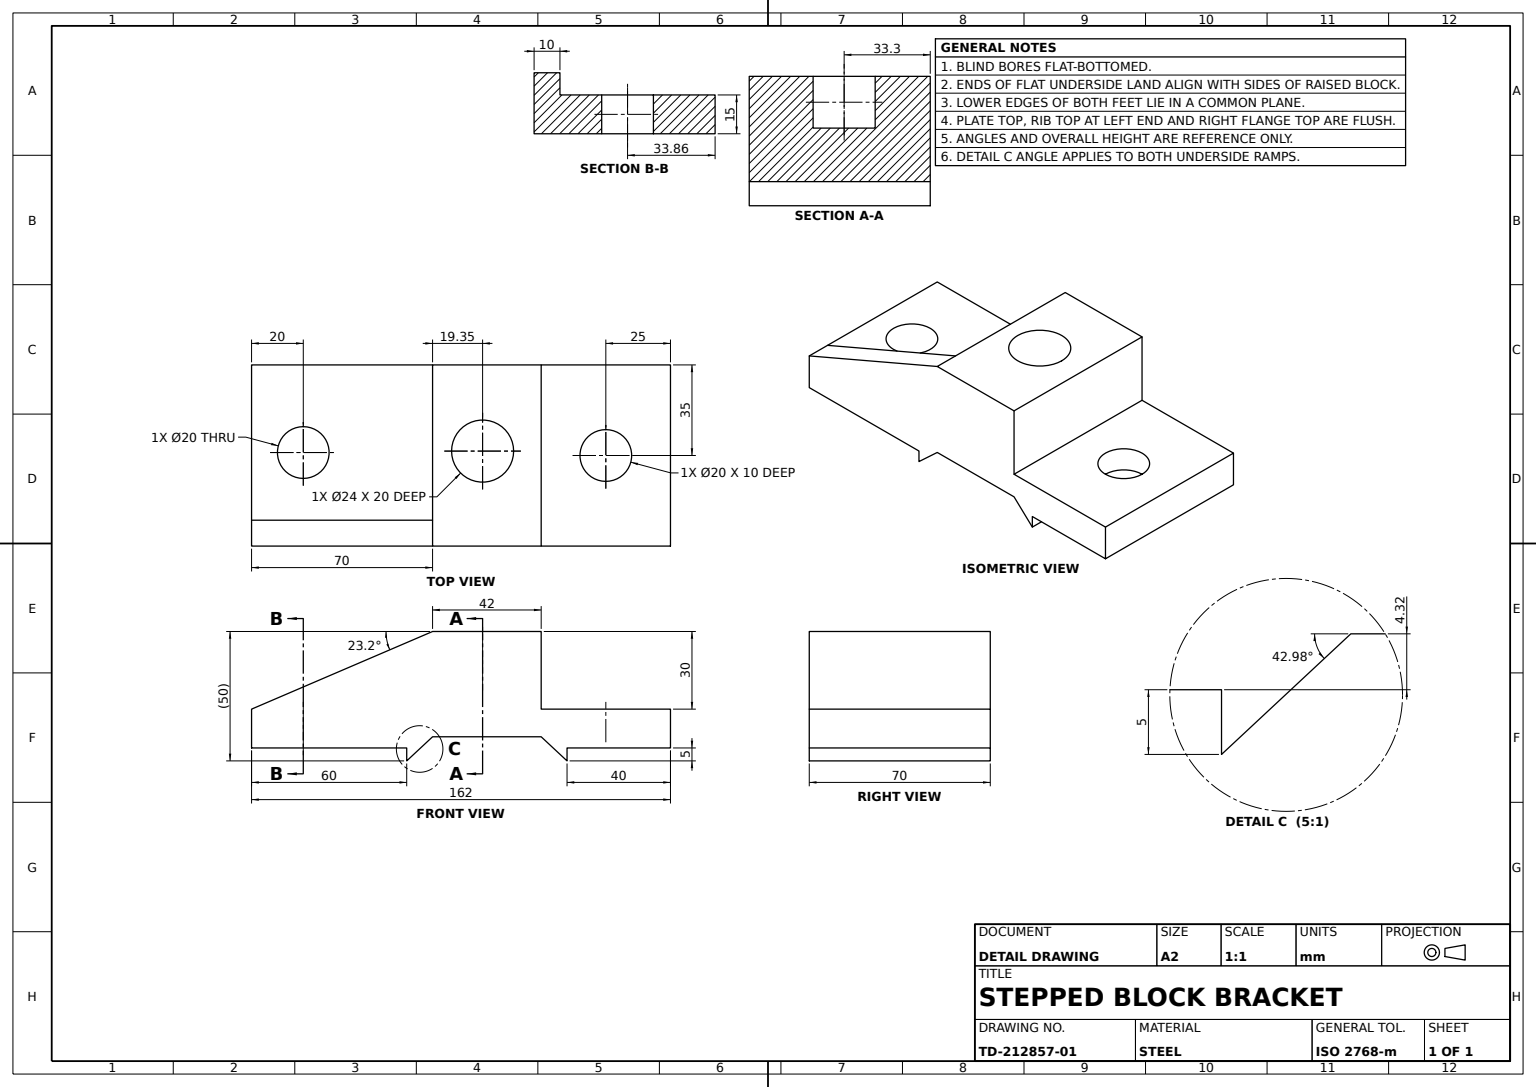
from build123d import *

# Parameters (mm, degrees)
STEPPED_BLOCK_BODY_DEPTH = 70
HOLE_A_SKETCH_R          = 10
HOLE_A_DEPTH_20_DEPTH    = 20
HOLE_B_SKETCH_R          = 12
HOLE_B_DEPTH_20_DEPTH    = 20
TRIANGULAR_LUG_DEPTH     = 10
ROUND_BOSS_SKETCH_R      = 10
ROUND_BOSS_10MM_DEPTH    = 10
HOLE_C_SKETCH_R          = 10
HOLE_C_DEPTH_10_DEPTH    = 10


with BuildPart() as part:
    # Stepped Block Profile Sketch → Stepped Block Body (new body)
    with BuildSketch(Plane.XY):
        Polygon((70, 0), (70, -5), (80, 4.319056963), (122, 4.319056963), (132, -5), (132, 0), (172, 0), (172, 15), (122, 15), (122, 45), (80, 45), (80, 15), (10, 15), (10, 0), align=None)
    extrude(amount=STEPPED_BLOCK_BODY_DEPTH)

    # Hole A Sketch → Hole A Depth 20 (cut)
    with BuildSketch(Plane(origin=(0, 15, 0), x_dir=(1, 0, 0), z_dir=(0, 1, 0))):
        with Locations(Location((30, -33.856567252, 0), (0, 0, 270))):
            Circle(HOLE_A_SKETCH_R)
    extrude(amount=-HOLE_A_DEPTH_20_DEPTH, mode=Mode.SUBTRACT)

    # Hole B Sketch → Hole B Depth 20 (cut)
    with BuildSketch(Plane(origin=(0, 45, 0), x_dir=(1, 0, 0), z_dir=(0, 1, 0))):
        with Locations(Location((99.347169036, -33.296354443, 0), (0, 0, 180))):
            Circle(HOLE_B_SKETCH_R)
    extrude(amount=-HOLE_B_DEPTH_20_DEPTH, mode=Mode.SUBTRACT)

    # Triangular Lug Sketch → Triangular Lug (add)
    with BuildSketch(Plane.XY.offset(70)):
        Polygon((10, 15), (80, 15), (80, 45), align=None)
    extrude(amount=-TRIANGULAR_LUG_DEPTH)

    # Round Boss Sketch → Round Boss 10mm (add)
    with BuildSketch(Plane(origin=(0, 15, 0), x_dir=(1, 0, 0), z_dir=(0, 1, 0))):
        with Locations((147.541656159, -38.188385292)):
            Circle(ROUND_BOSS_SKETCH_R)
    extrude(amount=-ROUND_BOSS_10MM_DEPTH)

    # Hole C Sketch → Hole C Depth 10 (cut)
    with BuildSketch(Plane(origin=(0, 15, 0), x_dir=(1, 0, 0), z_dir=(0, 1, 0))):
        with Locations(Location((147, -35, 0), (0, 0, 270))):
            Circle(HOLE_C_SKETCH_R)
    extrude(amount=-HOLE_C_DEPTH_10_DEPTH, mode=Mode.SUBTRACT)


solid = part.part
